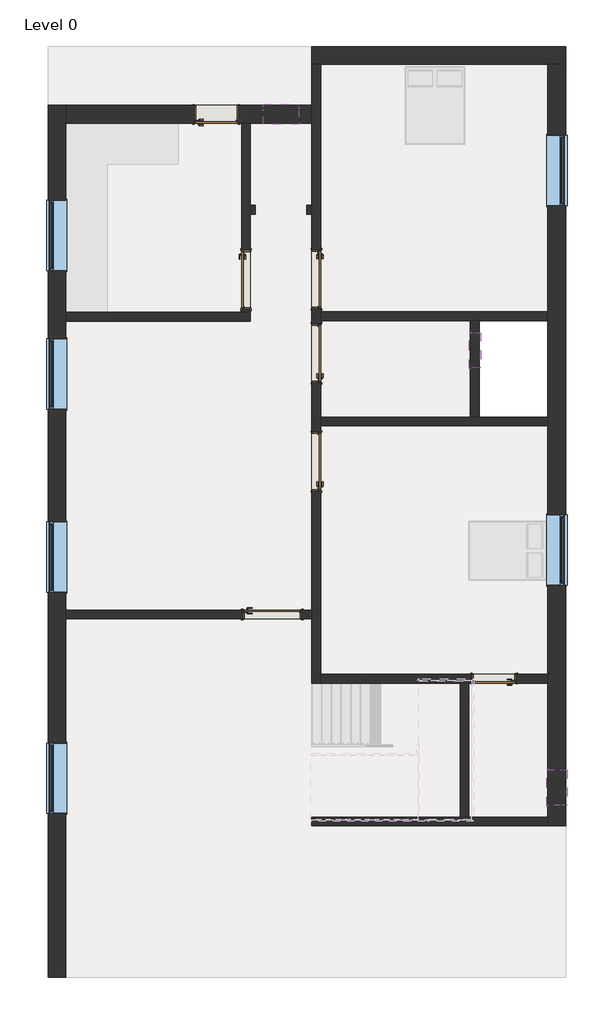
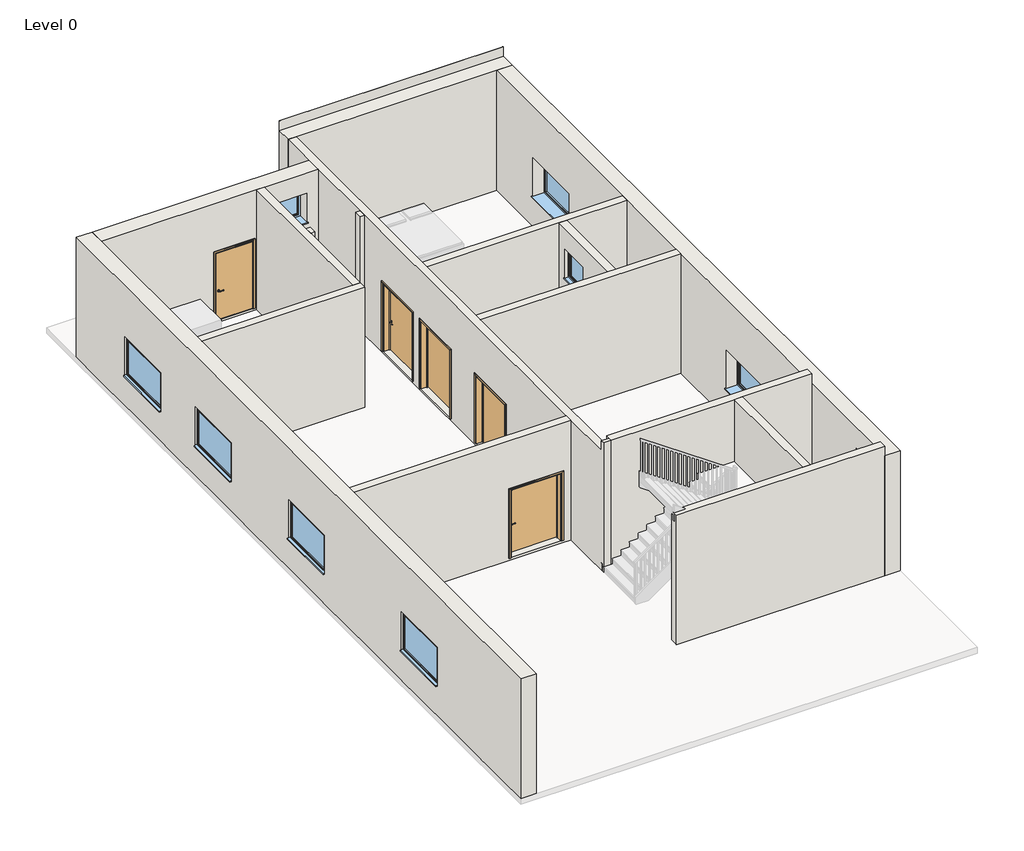
# One storey, part 1 of 2: 16 walls, 9 windows, 7 doors.
"""IFC4 building model written with IfcOpenShell, lengths in millimetres."""

from ifc_helpers import new_model, si_unit, frame, origin, origin_with_axes, place, context, project, spatial, polyline, outline, extrude, faceted_brep, transform, mapped, element, save
from components import doors_intsgl_d1_5c0f405e, doors_intsgl_d1_52b86bcf, doors_intsgl_d2_df50d10e, doors_intsgl_d2_875133e6, windows_sgl_plain_1810x1210mm_33e58113, windows_sgl_plain_1810x1210mm_8b4574cd, windows_sgl_plain_910x910mm_4715da24, windows_sgl_plain_910x910mm_27dc79fa, windows_sgl_plain_910x910mm_ba4b8fff

model = new_model("IFC4")

# Units and contexts
model_context = context("Model", 3, world=origin())
ifc_project = project(units=[si_unit("LENGTHUNIT", "METRE", prefix="MILLI")], contexts=[model_context])

# Site, building, storey
site = spatial("IfcSite", under=ifc_project)
building = spatial("IfcBuilding", under=site)
storey = spatial("IfcBuildingStorey", under=building, Name="Level 0", Elevation=0.0)

# Doors
placement = place(None, origin())
doors_intsgl_d1_shape = doors_intsgl_d1_5c0f405e(model_context)
element("IfcDoor", 1, ObjectType="Doors_IntSgl : D1", at=placement, inside=storey, context=model_context, shape_type="MappedRepresentation", body=[
    mapped(doors_intsgl_d1_shape, transform((-408.6988863, 5844.3566744, 76.2), x_axis=(0.0, -1.0, 0.0), y_axis=(1.0, 0.0, 0.0), z_axis=(0.0, 0.0, 1.0))),
])
element("IfcDoor", 2, ObjectType="Doors_IntSgl : D1", at=placement, inside=storey, context=model_context, shape_type="MappedRepresentation", body=[
    mapped(doors_intsgl_d1_shape, transform((-1538.9988863, -2784.8352742, 76.2), x_axis=(1.0, 0.0, 0.0), y_axis=(0.0, 1.0, 0.0), z_axis=(0.0, 0.0, 1.0))),
])
doors_intsgl_d1_2_shape = doors_intsgl_d1_52b86bcf(model_context)
element("IfcDoor", 3, ObjectType="Doors_IntSgl : D1", at=placement, inside=storey, context=model_context, shape_type="MappedRepresentation", body=[
    mapped(doors_intsgl_d1_2_shape, transform((-2218.4488863, 5838.4647258, 76.2), x_axis=(0.0, -1.0, 0.0), y_axis=(1.0, 0.0, 0.0), z_axis=(0.0, 0.0, 1.0))),
])
element("IfcDoor", 4, ObjectType="Doors_IntSgl : D1", at=placement, inside=storey, context=model_context, shape_type="MappedRepresentation", body=[
    mapped(doors_intsgl_d1_2_shape, transform((-408.6988863, 3939.3566744, 76.2), x_axis=(0.0, 1.0, 0.0), y_axis=(-1.0, 0.0, 0.0), z_axis=(0.0, 0.0, 1.0))),
])
element("IfcDoor", 5, ObjectType="Doors_IntSgl : D1", at=placement, inside=storey, context=model_context, shape_type="MappedRepresentation", body=[
    mapped(doors_intsgl_d1_2_shape, transform((-408.6988863, 1153.7809218, 76.2), x_axis=(0.0, 1.0, 0.0), y_axis=(-1.0, 0.0, 0.0), z_axis=(0.0, 0.0, 1.0))),
])
doors_intsgl_d2_shape = doors_intsgl_d2_df50d10e(model_context)
element("IfcDoor", 6, ObjectType="Doors_IntSgl : D2", at=placement, inside=storey, context=model_context, shape_type="MappedRepresentation", body=[
    mapped(doors_intsgl_d2_shape, transform((4169.6511137, -4435.8352742, 76.2), x_axis=(-1.0, 0.0, 0.0), y_axis=(0.0, -1.0, 0.0), z_axis=(0.0, 0.0, 1.0))),
])
doors_intsgl_d2_2_shape = doors_intsgl_d2_875133e6(model_context)
element("IfcDoor", 7, ObjectType="Doors_IntSgl : D2", at=placement, inside=storey, context=model_context, shape_type="MappedRepresentation", body=[
    mapped(doors_intsgl_d2_2_shape, transform((-2980.4488863, 10092.9647258, 76.2), x_axis=(1.0, 0.0, 0.0), y_axis=(0.0, 1.0, 0.0), z_axis=(0.0, 0.0, 1.0))),
])

# Walls
element("IfcWall", 8, ObjectType="EX WALL", at=placement, inside=storey, context=model_context, shape_type="Brep", body=[
    faceted_brep([(-7317.4988863, 10321.5647258, 0.0), (-7317.4988863, -12132.0352742, 0.0), (-7317.4988863, -12132.0352742, 3700.0), (-7317.4988863, 10321.5647258, 3700.0), (-7317.4988863, 7877.0647258, 2110.0), (-7317.4988863, 6067.0647258, 2110.0), (-7317.4988863, 6067.0647258, 900.0), (-7317.4988863, 7877.0647258, 900.0), (-7317.4988863, 4314.4647258, 2110.0), (-7317.4988863, 2504.4647258, 2110.0), (-7317.4988863, 2504.4647258, 900.0), (-7317.4988863, 4314.4647258, 900.0), (-7317.4988863, -403.3352742, 2110.0), (-7317.4988863, -2213.3352742, 2110.0), (-7317.4988863, -2213.3352742, 900.0), (-7317.4988863, -403.3352742, 900.0), (-7317.4988863, -6099.5352742, 2110.0), (-7317.4988863, -7909.5352742, 2110.0), (-7317.4988863, -7909.5352742, 900.0), (-7317.4988863, -6099.5352742, 900.0), (-6860.2988863, 10321.5647258, 0.0), (-6860.2988863, 10321.5647258, 3700.0), (-6860.2988863, 9864.3647258, 3700.0), (-6860.2988863, 5000.2647258, 3700.0), (-6860.2988863, 4771.6647258, 3700.0), (-6860.2988863, -2670.5352742, 3700.0), (-6860.2988863, -2899.1352742, 3700.0), (-6860.2988863, -12132.0352742, 3700.0), (-6860.2988863, -12132.0352742, 0.0), (-6860.2988863, -2899.1352742, 0.0), (-6860.2988863, -2670.5352742, 0.0), (-6860.2988863, 4771.6647258, 0.0), (-6860.2988863, 5000.2647258, 0.0), (-6860.2988863, 9864.3647258, 0.0), (-6860.2988863, 7877.0647258, 2110.0), (-6860.2988863, 7877.0647258, 900.0), (-6860.2988863, 6067.0647258, 900.0), (-6860.2988863, 6067.0647258, 2110.0), (-6860.2988863, 4314.4647258, 2110.0), (-6860.2988863, 4314.4647258, 900.0), (-6860.2988863, 2504.4647258, 900.0), (-6860.2988863, 2504.4647258, 2110.0), (-6860.2988863, -403.3352742, 2110.0), (-6860.2988863, -403.3352742, 900.0), (-6860.2988863, -2213.3352742, 900.0), (-6860.2988863, -2213.3352742, 2110.0), (-6860.2988863, -6099.5352742, 2110.0), (-6860.2988863, -6099.5352742, 900.0), (-6860.2988863, -7909.5352742, 900.0), (-6860.2988863, -7909.5352742, 2110.0)], [[[0, 1, 2, 3], [4, 5, 6, 7], [8, 9, 10, 11], [12, 13, 14, 15], [16, 17, 18, 19]], [[20, 21, 22, 23, 24, 25, 26, 27, 28, 29, 30, 31, 32, 33], [34, 35, 36, 37], [38, 39, 40, 41], [42, 43, 44, 45], [46, 47, 48, 49]], [[1, 0, 20, 33, 32, 31, 30, 29, 28]], [[2, 1, 28, 27]], [[0, 3, 21, 20]], [[3, 2, 27, 26, 25, 24, 23, 22, 21]], [[35, 34, 4, 7]], [[36, 35, 7, 6]], [[37, 36, 6, 5]], [[34, 37, 5, 4]], [[39, 38, 8, 11]], [[40, 39, 11, 10]], [[41, 40, 10, 9]], [[38, 41, 9, 8]], [[43, 42, 12, 15]], [[44, 43, 15, 14]], [[45, 44, 14, 13]], [[42, 45, 13, 12]], [[47, 46, 16, 19]], [[48, 47, 19, 18]], [[49, 48, 18, 17]], [[46, 49, 17, 16]]]),
])
element("IfcWall", 9, ObjectType="EX WALL", at=placement, inside=storey, context=model_context, shape_type="Brep", body=[
    faceted_brep([(-6860.2988863, 9864.3647258, 0.0), (-2332.7488863, 9864.3647258, 0.0), (-2104.1488863, 9864.3647258, 0.0), (-522.9988863, 9864.3647258, 0.0), (-522.9988863, 9864.3647258, 3700.0), (-2104.1488863, 9864.3647258, 3700.0), (-2332.7488863, 9864.3647258, 3700.0), (-6860.2988863, 9864.3647258, 3700.0), (-2408.9488863, 9864.3647258, 2186.2), (-2408.9488863, 9864.3647258, 76.2), (-3551.9488863, 9864.3647258, 76.2), (-3551.9488863, 9864.3647258, 2186.2), (-858.5738863, 9864.3647258, 3069.0), (-858.5738863, 9864.3647258, 2159.0), (-1768.5738863, 9864.3647258, 2159.0), (-1768.5738863, 9864.3647258, 3069.0), (-522.9988863, 10321.5647258, 0.0), (-6860.2988863, 10321.5647258, 0.0), (-6860.2988863, 10321.5647258, 3700.0), (-522.9988863, 10321.5647258, 3700.0), (-2408.9488863, 10321.5647258, 76.2), (-2408.9488863, 10321.5647258, 2186.2), (-3551.9488863, 10321.5647258, 2186.2), (-3551.9488863, 10321.5647258, 76.2), (-858.5738863, 10321.5647258, 3069.0), (-1768.5738863, 10321.5647258, 3069.0), (-1768.5738863, 10321.5647258, 2159.0), (-858.5738863, 10321.5647258, 2159.0)], [[[0, 1, 2, 3, 4, 5, 6, 7], [8, 9, 10, 11], [12, 13, 14, 15]], [[16, 17, 18, 19], [20, 21, 22, 23], [24, 25, 26, 27]], [[3, 2, 1, 0, 17, 16]], [[0, 7, 18, 17]], [[4, 3, 16, 19]], [[20, 9, 8, 21]], [[21, 8, 11, 22]], [[22, 11, 10, 23]], [[9, 20, 23, 10]], [[7, 6, 5, 4, 19, 18]], [[13, 12, 24, 27]], [[14, 13, 27, 26]], [[15, 14, 26, 25]], [[12, 15, 25, 24]]]),
])
element("IfcWall", 10, ObjectType="EX WALL", at=placement, inside=storey, context=model_context, shape_type="Brep", body=[
    faceted_brep([(-522.9988863, 11382.0147258, 0.0), (-294.3988863, 11382.0147258, 0.0), (5553.9511137, 11382.0147258, 0.0), (6011.1511137, 11382.0147258, 0.0), (6011.1511137, 11382.0147258, 3700.0), (5553.9511137, 11382.0147258, 3700.0), (-294.3988863, 11382.0147258, 3700.0), (-522.9988863, 11382.0147258, 3700.0), (-522.9988863, 11839.2147258, 0.0), (-522.9988863, 11839.2147258, 4000.0), (6011.1511137, 11839.2147258, 4000.0), (6011.1511137, 11839.2147258, 0.0), (6011.1511137, 11833.2891038, 4000.0), (6011.1511137, 11833.2891038, 3700.0), (-522.9988863, 11833.2891038, 3700.0), (-522.9988863, 11833.2891038, 4000.0)], [[[0, 1, 2, 3, 4, 5, 6, 7]], [[8, 9, 10, 11]], [[3, 2, 1, 0, 8, 11]], [[4, 3, 11, 10, 12, 13]], [[0, 7, 14, 15, 9, 8]], [[12, 10, 9, 15]], [[12, 15, 14, 13]], [[7, 6, 5, 4, 13, 14]]]),
])
element("IfcWall", 11, ObjectType="EX WALL", at=placement, inside=storey, context=model_context, shape_type="Brep", body=[
    faceted_brep([(5553.9511137, 11382.0147258, 0.0), (5553.9511137, 5006.1566744, 0.0), (5553.9511137, 4777.5566744, 0.0), (5553.9511137, 2296.7809218, 0.0), (5553.9511137, 2068.1809218, 0.0), (5553.9511137, -4321.5352742, 0.0), (5553.9511137, -4550.1352742, 0.0), (5553.9511137, -8002.321978, 0.0), (5553.9511137, -8230.921978, 0.0), (5553.9511137, -8230.921978, 3700.0), (5553.9511137, 2068.1809218, 3700.0), (5553.9511137, 2296.7809218, 3700.0), (5553.9511137, 4777.5566744, 3700.0), (5553.9511137, 5006.1566744, 3700.0), (5553.9511137, 11382.0147258, 3700.0), (5553.9511137, -2031.6771762, 2110.0), (5553.9511137, -2031.6771762, 900.0), (5553.9511137, -221.6771762, 900.0), (5553.9511137, -221.6771762, 2110.0), (5553.9511137, 9553.2147258, 2110.0), (5553.9511137, 7743.2147258, 2110.0), (5553.9511137, 7743.2147258, 900.0), (5553.9511137, 9553.2147258, 900.0), (5553.9511137, -6787.521978, 3069.0), (5553.9511137, -7697.521978, 3069.0), (5553.9511137, -7697.521978, 2159.0), (5553.9511137, -6787.521978, 2159.0), (6011.1511137, 11382.0147258, 0.0), (6011.1511137, 11382.0147258, 3700.0), (6011.1511137, -8230.921978, 3700.0), (6011.1511137, -8230.921978, 0.0), (6011.1511137, -2031.6771762, 2110.0), (6011.1511137, -221.6771762, 2110.0), (6011.1511137, -221.6771762, 900.0), (6011.1511137, -2031.6771762, 900.0), (6011.1511137, 9553.2147258, 2110.0), (6011.1511137, 9553.2147258, 900.0), (6011.1511137, 7743.2147258, 900.0), (6011.1511137, 7743.2147258, 2110.0), (6011.1511137, -6787.521978, 3069.0), (6011.1511137, -6787.521978, 2159.0), (6011.1511137, -7697.521978, 2159.0), (6011.1511137, -7697.521978, 3069.0)], [[[0, 1, 2, 3, 4, 5, 6, 7, 8, 9, 10, 11, 12, 13, 14], [15, 16, 17, 18], [19, 20, 21, 22], [23, 24, 25, 26]], [[27, 28, 29, 30], [31, 32, 33, 34], [35, 36, 37, 38], [39, 40, 41, 42]], [[8, 7, 6, 5, 4, 3, 2, 1, 0, 27, 30]], [[0, 14, 28, 27]], [[9, 8, 30, 29]], [[14, 13, 12, 11, 10, 9, 29, 28]], [[16, 15, 31, 34]], [[17, 16, 34, 33]], [[18, 17, 33, 32]], [[15, 18, 32, 31]], [[36, 35, 19, 22]], [[37, 36, 22, 21]], [[38, 37, 21, 20]], [[35, 38, 20, 19]], [[40, 39, 23, 26]], [[41, 40, 26, 25]], [[42, 41, 25, 24]], [[39, 42, 24, 23]]]),
])
element("IfcWall", 12, ObjectType="IN WALL", at=placement, inside=storey, context=model_context, shape_type="Brep", body=[
    faceted_brep([(-6860.2988863, 4771.6647258, 0.0), (-2104.1488863, 4771.6647258, 0.0), (-2104.1488863, 4771.6647258, 3700.0), (-6860.2988863, 4771.6647258, 3700.0), (-6860.2988863, 5000.2647258, 0.0), (-6860.2988863, 5000.2647258, 3700.0), (-2332.7488863, 5000.2647258, 3700.0), (-2104.1488863, 5000.2647258, 3700.0), (-2104.1488863, 5000.2647258, 0.0), (-2332.7488863, 5000.2647258, 0.0)], [[[0, 1, 2, 3]], [[4, 5, 6, 7, 8, 9]], [[1, 0, 4, 9, 8]], [[0, 3, 5, 4]], [[2, 1, 8, 7]], [[3, 2, 7, 6, 5]]]),
])
element("IfcWall", 13, ObjectType="IN WALL", at=placement, inside=storey, context=model_context, shape_type="Brep", body=[
    faceted_brep([(-2104.1488863, 5000.2647258, 0.0), (-2104.1488863, 7521.4694415, 0.0), (-2104.1488863, 7750.0694415, 0.0), (-2104.1488863, 9864.3647258, 0.0), (-2104.1488863, 9864.3647258, 3700.0), (-2104.1488863, 7750.0694415, 3700.0), (-2104.1488863, 7521.4694415, 3700.0), (-2104.1488863, 5000.2647258, 3700.0), (-2104.1488863, 5076.4647258, 76.2), (-2104.1488863, 5076.4647258, 2186.2), (-2104.1488863, 6600.4647258, 2186.2), (-2104.1488863, 6600.4647258, 76.2), (-2332.7488863, 9864.3647258, 0.0), (-2332.7488863, 5000.2647258, 0.0), (-2332.7488863, 5000.2647258, 3700.0), (-2332.7488863, 9864.3647258, 3700.0), (-2332.7488863, 5076.4647258, 2186.2), (-2332.7488863, 5076.4647258, 76.2), (-2332.7488863, 6600.4647258, 76.2), (-2332.7488863, 6600.4647258, 2186.2)], [[[0, 1, 2, 3, 4, 5, 6, 7], [8, 9, 10, 11]], [[12, 13, 14, 15], [16, 17, 18, 19]], [[3, 2, 1, 0, 13, 12]], [[0, 7, 14, 13]], [[4, 3, 12, 15]], [[8, 17, 16, 9]], [[9, 16, 19, 10]], [[10, 19, 18, 11]], [[17, 8, 11, 18]], [[7, 6, 5, 4, 15, 14]]]),
])
element("IfcWall", 14, ObjectType="IN WALL", at=placement, inside=storey, context=model_context, shape_type="Brep", body=[
    faceted_brep([(-522.9988863, 11382.0147258, 0.0), (-522.9988863, 10321.5647258, 0.0), (-522.9988863, 9864.3647258, 0.0), (-522.9988863, 7750.0694415, 0.0), (-522.9988863, 7521.4694415, 0.0), (-522.9988863, -2670.5352742, 0.0), (-522.9988863, -2899.1352742, 0.0), (-522.9988863, -4550.1352742, 0.0), (-522.9988863, -4550.1352742, 4000.0), (-522.9988863, -4436.6352742, 4000.0), (-522.9988863, -4436.6352742, 3700.0), (-522.9988863, -2899.1352742, 3700.0), (-522.9988863, -2670.5352742, 3700.0), (-522.9988863, 7521.4694415, 3700.0), (-522.9988863, 7750.0694415, 3700.0), (-522.9988863, 9864.3647258, 3700.0), (-522.9988863, 10321.5647258, 3700.0), (-522.9988863, 11382.0147258, 3700.0), (-522.9988863, 5082.3566744, 2186.2), (-522.9988863, 5082.3566744, 76.2), (-522.9988863, 6606.3566744, 76.2), (-522.9988863, 6606.3566744, 2186.2), (-522.9988863, 4701.3566744, 76.2), (-522.9988863, 4701.3566744, 2186.2), (-522.9988863, 3177.3566744, 2186.2), (-522.9988863, 3177.3566744, 76.2), (-522.9988863, 1915.7809218, 76.2), (-522.9988863, 1915.7809218, 2186.2), (-522.9988863, 391.7809218, 2186.2), (-522.9988863, 391.7809218, 76.2), (-294.3988863, -4550.1352742, 0.0), (-294.3988863, -4321.5352742, 0.0), (-294.3988863, 2068.1809218, 0.0), (-294.3988863, 2296.7809218, 0.0), (-294.3988863, 4777.5566744, 0.0), (-294.3988863, 5006.1566744, 0.0), (-294.3988863, 11382.0147258, 0.0), (-294.3988863, 11382.0147258, 3700.0), (-294.3988863, 5006.1566744, 3700.0), (-294.3988863, 4777.5566744, 3700.0), (-294.3988863, 2296.7809218, 3700.0), (-294.3988863, 2068.1809218, 3700.0), (-294.3988863, -4436.6352742, 3700.0), (-294.3988863, -4436.6352742, 4000.0), (-294.3988863, -4550.1352742, 4000.0), (-294.3988863, 5082.3566744, 76.2), (-294.3988863, 5082.3566744, 2186.2), (-294.3988863, 6606.3566744, 2186.2), (-294.3988863, 6606.3566744, 76.2), (-294.3988863, 4701.3566744, 2186.2), (-294.3988863, 4701.3566744, 76.2), (-294.3988863, 3177.3566744, 76.2), (-294.3988863, 3177.3566744, 2186.2), (-294.3988863, 1915.7809218, 2186.2), (-294.3988863, 1915.7809218, 76.2), (-294.3988863, 391.7809218, 76.2), (-294.3988863, 391.7809218, 2186.2)], [[[0, 1, 2, 3, 4, 5, 6, 7, 8, 9, 10, 11, 12, 13, 14, 15, 16, 17], [18, 19, 20, 21], [22, 23, 24, 25], [26, 27, 28, 29]], [[30, 31, 32, 33, 34, 35, 36, 37, 38, 39, 40, 41, 42, 43, 44], [45, 46, 47, 48], [49, 50, 51, 52], [53, 54, 55, 56]], [[7, 6, 5, 4, 3, 2, 1, 0, 36, 35, 34, 33, 32, 31, 30]], [[0, 17, 37, 36]], [[8, 7, 30, 44]], [[45, 19, 18, 46]], [[46, 18, 21, 47]], [[47, 21, 20, 48]], [[19, 45, 48, 20]], [[23, 22, 50, 49]], [[24, 23, 49, 52]], [[25, 24, 52, 51]], [[22, 25, 51, 50]], [[27, 26, 54, 53]], [[28, 27, 53, 56]], [[29, 28, 56, 55]], [[26, 29, 55, 54]], [[8, 44, 43, 9]], [[9, 43, 42, 10]], [[37, 17, 16, 15, 14, 13, 12, 11, 10, 42, 41, 40, 39, 38]]]),
])
element("IfcWall", 15, ObjectType="IN WALL", at=placement, inside=storey, context=model_context, shape_type="Brep", body=[
    faceted_brep([(-294.3988863, -4550.1352742, 0.0), (3293.3511137, -4550.1352742, 0.0), (3521.9511137, -4550.1352742, 0.0), (5553.9511137, -4550.1352742, 0.0), (5553.9511137, -4550.1352742, 4000.0), (3521.6011137, -4550.1352742, 4000.0), (3293.3511137, -4550.1352742, 4000.0), (-294.3988863, -4550.1352742, 4000.0), (3598.1511137, -4550.1352742, 76.2), (3598.1511137, -4550.1352742, 2186.2), (4741.1511137, -4550.1352742, 2186.2), (4741.1511137, -4550.1352742, 76.2), (5553.9511137, -4321.5352742, 0.0), (-294.3988863, -4321.5352742, 0.0), (-294.3988863, -4321.5352742, 4000.0), (5553.9511137, -4321.5352742, 4000.0), (3598.1511137, -4321.5352742, 2186.2), (3598.1511137, -4321.5352742, 76.2), (4741.1511137, -4321.5352742, 76.2), (4741.1511137, -4321.5352742, 2186.2), (-294.3988863, -4436.6352742, 4000.0)], [[[0, 1, 2, 3, 4, 5, 6, 7], [8, 9, 10, 11]], [[12, 13, 14, 15], [16, 17, 18, 19]], [[3, 2, 1, 0, 13, 12]], [[7, 6, 5, 4, 15, 14, 20]], [[0, 7, 20, 14, 13]], [[4, 3, 12, 15]], [[8, 17, 16, 9]], [[9, 16, 19, 10]], [[10, 19, 18, 11]], [[17, 8, 11, 18]]]),
])
element("IfcWall", 16, ObjectType="IN WALL", at=placement, inside=storey, context=model_context, shape_type="Brep", body=[
    faceted_brep([(-520.2140986, -8230.921978, 0.0), (5553.9511137, -8230.921978, 0.0), (5553.9511137, -8230.921978, 3700.0), (5553.9511137, -8230.921978, 4000.0), (-520.2140986, -8230.921978, 4000.0), (-520.2140986, -8002.321978, 0.0), (-520.2140986, -8002.321978, 4000.0), (3293.3511137, -8002.321978, 4000.0), (3521.6011137, -8002.321978, 4000.0), (5553.9511137, -8002.321978, 4000.0), (5553.9511137, -8002.321978, 0.0), (3521.9511137, -8002.321978, 0.0), (3293.3511137, -8002.321978, 0.0)], [[[0, 1, 2, 3, 4]], [[5, 6, 7, 8, 9, 10, 11, 12]], [[1, 0, 5, 12, 11, 10]], [[4, 3, 9, 8, 7, 6]], [[0, 4, 6, 5]], [[3, 2, 1, 10, 9]]]),
])
element("IfcWall", 17, ObjectType="IN WALL", at=placement, inside=storey, context=model_context, shape_type="SweptSolid", body=[
    extrude(outline(polyline([(4000.0, 3293.3511137), (0.0, 3293.3511137), (0.0, 3521.9511137), (3700.0, 3521.9511137), (3700.0, 3521.6011137), (4000.0, 3521.6011137), (4000.0, 3293.3511137)])), frame((0.0, -8002.321978, 0.0), z_axis=(0.0, 1.0, 0.0), x_axis=(0.0, 0.0, 1.0)), (0.0, 0.0, 1.0), 3452.1867039),
])
element("IfcWall", 18, ObjectType="IN WALL", at=placement, inside=storey, context=model_context, shape_type="SweptSolid", body=[
    extrude(outline(polyline([(0.0, -6860.2988863), (0.0, -522.9988863), (3700.0, -522.9988863), (3700.0, -6860.2988863), (0.0, -6860.2988863)]), holes=[polyline([(2186.2, -776.9988863), (76.2, -776.9988863), (76.2, -2300.9988863), (2186.2, -2300.9988863), (2186.2, -776.9988863)])]), frame((0.0, -2899.1352742, 0.0), z_axis=(0.0, 1.0, 0.0), x_axis=(0.0, 0.0, 1.0)), (0.0, 0.0, 1.0), 228.6),
])
element("IfcWall", 19, ObjectType="IN WALL", at=placement, inside=storey, context=model_context, shape_type="Brep", body=[
    faceted_brep([(-294.3988863, 4777.5566744, 0.0), (3560.0511137, 4777.5566744, 0.0), (3788.6511137, 4777.5566744, 0.0), (5553.9511137, 4777.5566744, 0.0), (5553.9511137, 4777.5566744, 3700.0), (3788.6511137, 4777.5566744, 3700.0), (3560.0511137, 4777.5566744, 3700.0), (-294.3988863, 4777.5566744, 3700.0), (-294.3988863, 5006.1566744, 0.0), (-294.3988863, 5006.1566744, 3700.0), (5553.9511137, 5006.1566744, 3700.0), (5553.9511137, 5006.1566744, 0.0)], [[[0, 1, 2, 3, 4, 5, 6, 7]], [[8, 9, 10, 11]], [[3, 2, 1, 0, 8, 11]], [[4, 3, 11, 10]], [[0, 7, 9, 8]], [[7, 6, 5, 4, 10, 9]]]),
])
element("IfcWall", 20, ObjectType="IN WALL", at=placement, inside=storey, context=model_context, shape_type="Brep", body=[
    faceted_brep([(-294.3988863, 2068.1809218, 0.0), (5553.9511137, 2068.1809218, 0.0), (5553.9511137, 2068.1809218, 3700.0), (-294.3988863, 2068.1809218, 3700.0), (-294.3988863, 2296.7809218, 0.0), (-294.3988863, 2296.7809218, 3700.0), (3560.0511137, 2296.7809218, 3700.0), (3788.6511137, 2296.7809218, 3700.0), (5553.9511137, 2296.7809218, 3700.0), (5553.9511137, 2296.7809218, 0.0), (3788.6511137, 2296.7809218, 0.0), (3560.0511137, 2296.7809218, 0.0)], [[[0, 1, 2, 3]], [[4, 5, 6, 7, 8, 9, 10, 11]], [[1, 0, 4, 11, 10, 9]], [[2, 1, 9, 8]], [[0, 3, 5, 4]], [[3, 2, 8, 7, 6, 5]]]),
])
element("IfcWall", 21, ObjectType="IN WALL", at=placement, inside=storey, context=model_context, shape_type="SweptSolid", body=[
    extrude(outline(polyline([(4777.5566744, 0.0), (2296.7809218, 0.0), (2296.7809218, 3700.0), (4777.5566744, 3700.0), (4777.5566744, 0.0)]), holes=[polyline([(4472.7566744, 3069.0), (3562.7566744, 3069.0), (3562.7566744, 2159.0), (4472.7566744, 2159.0), (4472.7566744, 3069.0)])]), frame((3560.0511137, 0.0, 0.0), z_axis=(1.0, 0.0, 0.0), x_axis=(0.0, 1.0, 0.0)), (0.0, 0.0, 1.0), 228.6),
])
element("IfcWall", 22, ObjectType="IN WALL", at=placement, inside=storey, context=model_context, shape_type="SweptSolid", body=[
    extrude(outline(polyline([(-1977.1488863, 7521.4694415), (-2104.1488863, 7521.4694415), (-2104.1488863, 7750.0694415), (-1977.1488863, 7750.0694415), (-1977.1488863, 7521.4694415)])), origin_with_axes(), (0.0, 0.0, 1.0), 3700.0),
])
element("IfcWall", 23, ObjectType="IN WALL", at=placement, inside=storey, context=model_context, shape_type="SweptSolid", body=[
    extrude(outline(polyline([(-522.9988863, 7521.4694415), (-649.9988863, 7521.4694415), (-649.9988863, 7750.0694415), (-522.9988863, 7750.0694415), (-522.9988863, 7521.4694415)])), origin_with_axes(), (0.0, 0.0, 1.0), 3700.0),
])

# Windows
windows_sgl_plain_1810x1210mm_shape = windows_sgl_plain_1810x1210mm_33e58113(model_context)
element("IfcWindow", 24, ObjectType="Windows_Sgl_Plain : 1810x1210mm", at=placement, inside=storey, context=model_context, shape_type="MappedRepresentation", body=[
    mapped(windows_sgl_plain_1810x1210mm_shape, transform((5774.0945459, 8648.2147258, 0.0), x_axis=(0.0, -1.0, 0.0), y_axis=(1.0, 0.0, 0.0), z_axis=(0.0, 0.0, 1.0))),
])
windows_sgl_plain_1810x1210mm_2_shape = windows_sgl_plain_1810x1210mm_8b4574cd(model_context)
element("IfcWindow", 25, ObjectType="Windows_Sgl_Plain : 1810x1210mm", at=placement, inside=storey, context=model_context, shape_type="MappedRepresentation", body=[
    mapped(windows_sgl_plain_1810x1210mm_2_shape, transform((-7080.4423185, 6972.0647258, 0.0), x_axis=(0.0, -1.0, 0.0), y_axis=(1.0, 0.0, 0.0), z_axis=(0.0, 0.0, 1.0))),
])
element("IfcWindow", 26, ObjectType="Windows_Sgl_Plain : 1810x1210mm", at=placement, inside=storey, context=model_context, shape_type="MappedRepresentation", body=[
    mapped(windows_sgl_plain_1810x1210mm_2_shape, transform((-7080.4423185, 3409.4647258, 0.0), x_axis=(0.0, -1.0, 0.0), y_axis=(1.0, 0.0, 0.0), z_axis=(0.0, 0.0, 1.0))),
])
element("IfcWindow", 27, ObjectType="Windows_Sgl_Plain : 1810x1210mm", at=placement, inside=storey, context=model_context, shape_type="MappedRepresentation", body=[
    mapped(windows_sgl_plain_1810x1210mm_2_shape, transform((-7080.4423185, -1308.3352742, 0.0), x_axis=(0.0, -1.0, 0.0), y_axis=(1.0, 0.0, 0.0), z_axis=(0.0, 0.0, 1.0))),
])
element("IfcWindow", 28, ObjectType="Windows_Sgl_Plain : 1810x1210mm", at=placement, inside=storey, context=model_context, shape_type="MappedRepresentation", body=[
    mapped(windows_sgl_plain_1810x1210mm_2_shape, transform((-7080.4423185, -7004.5352742, 0.0), x_axis=(0.0, -1.0, 0.0), y_axis=(1.0, 0.0, 0.0), z_axis=(0.0, 0.0, 1.0))),
])
element("IfcWindow", 29, ObjectType="Windows_Sgl_Plain : 1810x1210mm", at=placement, inside=storey, context=model_context, shape_type="MappedRepresentation", body=[
    mapped(windows_sgl_plain_1810x1210mm_2_shape, transform((5774.0945459, -1126.6771762, 0.0), x_axis=(0.0, 1.0, 0.0), y_axis=(-1.0, 0.0, 0.0), z_axis=(0.0, 0.0, 1.0))),
])
windows_sgl_plain_910x910mm_shape = windows_sgl_plain_910x910mm_4715da24(model_context)
element("IfcWindow", 30, ObjectType="Windows_Sgl_Plain : 910x910mm", at=placement, inside=storey, context=model_context, shape_type="MappedRepresentation", body=[
    mapped(windows_sgl_plain_910x910mm_shape, transform((5774.0945459, -7242.521978, 959.0), x_axis=(0.0, -1.0, 0.0), y_axis=(1.0, 0.0, 0.0), z_axis=(0.0, 0.0, 1.0))),
])
windows_sgl_plain_910x910mm_2_shape = windows_sgl_plain_910x910mm_27dc79fa(model_context)
element("IfcWindow", 31, ObjectType="Windows_Sgl_Plain : 910x910mm", at=placement, inside=storey, context=model_context, shape_type="MappedRepresentation", body=[
    mapped(windows_sgl_plain_910x910mm_2_shape, transform((-1313.5738863, 10084.508158, 959.0), x_axis=(-1.0, 0.0, 0.0), y_axis=(0.0, -1.0, 0.0), z_axis=(0.0, 0.0, 1.0))),
])
windows_sgl_plain_910x910mm_3_shape = windows_sgl_plain_910x910mm_ba4b8fff(model_context)
element("IfcWindow", 32, ObjectType="Windows_Sgl_Plain : 910x910mm", at=placement, inside=storey, context=model_context, shape_type="MappedRepresentation", body=[
    mapped(windows_sgl_plain_910x910mm_3_shape, transform((3665.8945459, 4017.7566744, 959.0), x_axis=(0.0, -1.0, 0.0), y_axis=(1.0, 0.0, 0.0), z_axis=(0.0, 0.0, 1.0))),
])

save(model, "model.ifc")

# Revit data of these elements
# Type "Doors_IntSgl : D1"
#   Type Mark = "46"
#   Type Comments = "Internal Single"
#   Operation = "SingleSwingRight"
#   Manufacturer = "Revit"
#   Keynote = "L20"
#   Description = "Internal Single Door"
#   Analytic Construction = "Metal"
#   UnderCut = 8 mm
#   Tolerance = 2 mm
#   Thickness = 38 mm
#   Thermal Resistance (R) = 0.270117 (m²·K)/W
#   Structural Tolerance = 8 mm
#   StopDepth = 32 mm
#   Stop Thickness = 19 mm
#   Rough Width = 1524 mm
#   Rough Height = 2110 mm
#   Height to Top Lock Rail = 1000 mm
#   Heat Transfer Coefficient (U) = 3.7021 W/(m²·K)
#   Handle Z Distance = 900 mm
#   Handle X Distance = 75 mm
#   Frame Thickness = 32 mm
#   Door Panel Width = 1440 mm
#   Door Panel Thickness = 38 mm
#   Door Panel Offset = 0 mm
#   Height = 2110 mm
#   Width = 1524 mm
#   Door Panel Height = 2060 mm
#   Architrave Setback = 5 mm
#   Vis - Ironmongery = yes
#   Material Ironmongery = Door - Handle
#   Material Frame = Door - Frame/Mullion (1)
#   Material Door = Door - Panel
#   Material Architrave = Door - Architrave
#   Visual Light Transmittance = 0
#   Solar Heat Gain Coefficient = 0
#   Function = (empty or 0)
#   Wall Closure = (empty or 0)
# Type "Doors_IntSgl : D2"
#   Type Mark = "47"
#   Type Comments = "Internal Single"
#   Operation = "SingleSwingRight"
#   Manufacturer = "Revit"
#   Keynote = "L20"
#   Description = "Internal Single Door"
#   Analytic Construction = "Metal"
#   UnderCut = 8 mm
#   Tolerance = 2 mm
#   Thickness = 38 mm
#   Thermal Resistance (R) = 0.270117 (m²·K)/W
#   Structural Tolerance = 8 mm
#   StopDepth = 32 mm
#   Stop Thickness = 19 mm
#   Rough Width = 1143 mm
#   Rough Height = 2110 mm
#   Height to Top Lock Rail = 1000 mm
#   Heat Transfer Coefficient (U) = 3.7021 W/(m²·K)
#   Handle Z Distance = 900 mm
#   Handle X Distance = 75 mm
#   Frame Thickness = 32 mm
#   Door Panel Width = 1059 mm
#   Door Panel Thickness = 38 mm
#   Door Panel Offset = 0 mm
#   Height = 2110 mm
#   Width = 1143 mm
#   Door Panel Height = 2060 mm
#   Architrave Setback = 5 mm
#   Vis - Ironmongery = yes
#   Material Ironmongery = Door - Handle
#   Material Frame = Door - Frame/Mullion (1)
#   Material Door = Door - Panel
#   Material Architrave = Door - Architrave
#   Visual Light Transmittance = 0
#   Solar Heat Gain Coefficient = 0
#   Function = (empty or 0)
#   Wall Closure = (empty or 0)
# Type "EX WALL"
#   Keynote = "F10"
#   Layers, outside or top first: 457.2 mm "Concrete Masonry Units _Low Density" (function 1)
# Type "IN WALL"
#   Keynote = "F10"
#   Layers, outside or top first: 228.6 mm "Concrete Masonry Units _Low Density" (function 1)
# Type "Windows_Sgl_Plain : 1810x1210mm"
#   Type Mark = "49"
#   Operation = "SinglePanel"
#   Construction Type Id = "SGL"
#   Manufacturer = "Revit"
#   Keynote = "L10"
#   Analytic Construction = "Large single-glazed windows"
#   Wrap Layers (Ext) from Ext = 102.5 mm
#   Wrap Layers (Int) from Ext = 177.5 mm
#   Window Board Projection = 25 mm
#   Window Board Extension = 25 mm
#   Visual Light Transmittance = 0.9
#   Solar Heat Gain Coefficient = 0.86
#   Rough Width = 1810 mm
#   Rough Height = 1210 mm
#   Height = 1210 mm
#   Width = 1810 mm
#   Heat Transfer Coefficient (U) = 5.5617 W/(m²·K)
#   Glazing Thickness = 24 mm
#   FrameOffset - External = 50 mm
#   Frame Depth = 65 mm
#   Default Head Height = 2110 mm
#   Cill Depth = 87.5 mm
#   Cavity Closer Width = 50 mm
#   Cavity Closer Offset from Ext = 102.5 mm
#   Cavity Closer Depth = 85 mm
#   Define Thermal Properties by = 1
#   Vis - Cavity Closers = yes
#   Define Thermal Properties by = 1
#   Material Trim = Window Frame
#   Material Glass = Glass
#   Material Frame = Window Frame
#   Wall Closure = (empty or 0)
# Type "Windows_Sgl_Plain : 910x910mm"
#   Type Mark = "44"
#   Operation = "SinglePanel"
#   Construction Type Id = "SGL"
#   Manufacturer = "Revit"
#   Keynote = "L10"
#   Analytic Construction = "Large single-glazed windows"
#   Wrap Layers (Ext) from Ext = 102.5 mm
#   Wrap Layers (Int) from Ext = 177.5 mm
#   Window Board Projection = 25 mm
#   Window Board Extension = 25 mm
#   Visual Light Transmittance = 0.9
#   Solar Heat Gain Coefficient = 0.86
#   Rough Width = 910 mm
#   Rough Height = 910 mm
#   Height = 910 mm
#   Width = 910 mm
#   Heat Transfer Coefficient (U) = 5.5617 W/(m²·K)
#   Glazing Thickness = 24 mm
#   FrameOffset - External = 50 mm
#   Frame Depth = 65 mm
#   Default Head Height = 2110 mm
#   Cill Depth = 87.5 mm
#   Cavity Closer Width = 50 mm
#   Cavity Closer Offset from Ext = 102.5 mm
#   Cavity Closer Depth = 85 mm
#   Define Thermal Properties by = 1
#   Vis - Cavity Closers = yes
#   Define Thermal Properties by = 1
#   Material Trim = Window Frame
#   Material Glass = Glass
#   Material Frame = Window Frame
#   Wall Closure = (empty or 0)
# Elements 1, 2, 3, 4, 5 (IfcDoor, "Doors_IntSgl : D1")
#   Phase Created = New Construction
#   Materials on its faces: "Door - Architrave", "Door - Handle", "Door - Frame/Mullion (1)", "Door - Panel"
# Elements 6, 7 (IfcDoor, "Doors_IntSgl : D2")
#   Phase Created = New Construction
#   Materials on its faces: "Door - Architrave", "Door - Handle", "Door - Frame/Mullion (1)", "Door - Panel"
# Elements 8, 9, 10, 11 (IfcWall, "EX WALL")
#   Top Offset = 0 mm
#   Base Offset = 0 mm
#   wall height = 4000 mm
#   Phase Created = New Construction
#   Base Constraint = Level 0
#   Top Constraint = Level 1
#   Materials on its faces: "Concrete Masonry Units _Low Density"
# Elements 12, 13, 14, 15, 16, 17, 18, 19, 20, 21, 22, 23 (IfcWall, "IN WALL")
#   Top Offset = 0 mm
#   Base Offset = 0 mm
#   wall height = 4000 mm
#   Phase Created = New Construction
#   Base Constraint = Level 0
#   Top Constraint = Level 1
#   Materials on its faces: "Concrete Masonry Units _Low Density"
# Element 24 (IfcWindow, "Windows_Sgl_Plain : 1810x1210mm")
#   Mark = "6"
#   Phase Created = New Construction
#   Materials on its faces: "Window Frame", "Glass"
# Element 25 (IfcWindow, "Windows_Sgl_Plain : 1810x1210mm")
#   Mark = "1"
#   Phase Created = New Construction
#   Materials on its faces: "Window Frame", "Glass"
# Element 26 (IfcWindow, "Windows_Sgl_Plain : 1810x1210mm")
#   Mark = "2"
#   Phase Created = New Construction
#   Materials on its faces: "Window Frame", "Glass"
# Element 27 (IfcWindow, "Windows_Sgl_Plain : 1810x1210mm")
#   Mark = "3"
#   Phase Created = New Construction
#   Materials on its faces: "Window Frame", "Glass"
# Element 28 (IfcWindow, "Windows_Sgl_Plain : 1810x1210mm")
#   Mark = "4"
#   Phase Created = New Construction
#   Materials on its faces: "Window Frame", "Glass"
# Element 29 (IfcWindow, "Windows_Sgl_Plain : 1810x1210mm")
#   Mark = "5"
#   Phase Created = New Construction
#   Materials on its faces: "Window Frame", "Glass"
# Element 30 (IfcWindow, "Windows_Sgl_Plain : 910x910mm")
#   Mark = "8"
#   Phase Created = New Construction
#   Materials on its faces: "Window Frame", "Glass"
# Element 31 (IfcWindow, "Windows_Sgl_Plain : 910x910mm")
#   Mark = "7"
#   Phase Created = New Construction
#   Materials on its faces: "Window Frame", "Glass"
# Element 32 (IfcWindow, "Windows_Sgl_Plain : 910x910mm")
#   Mark = "9"
#   Phase Created = New Construction
#   Materials on its faces: "Window Frame", "Glass"
# Materials
#   "Door - Handle": colour RGB 0 0 0, transparency 0, Keynote = "P21", Cost = 0
#   "Door - Frame/Mullion (1)": class "Wood", colour RGB 212 179 113, transparency 0, Keynote = "L20", Cost = 0
#   "Door - Panel": class "Wood", colour RGB 210 159 95, transparency 0, Keynote = "L20", Cost = 0
#   "Door - Architrave": class "Wood", colour RGB 154 90 5, transparency 0, Keynote = "P20", Cost = 0
#   "Concrete Masonry Units _Low Density": class "Masonry", colour RGB 181 181 181, transparency 0, Description = "Concrete masonry units", Cost = 0
#   "Window Frame": colour RGB 249 249 249, transparency 0, Keynote = "L10", Cost = 0
#   "Glass": class "Glass", colour RGB 0 128 192, transparency 0.9, Description = "Soda Lime Glass", Cost = 0
# Room at (4545.224, -6189.837) mm, phase "New Construction", upper level "Level 0", upper offset 3999.992 mm, lower offset 0 mm
#   Number = "8"
#   Name = "toilet 2"
# Room at (-4313.75, 7572.957) mm, phase "New Construction", upper level "Level 0", upper offset 3999.992 mm, lower offset 0 mm
#   Number = "1"
#   Name = "kitchen"
# Room at (-3301.75, 945.757) mm, phase "New Construction", upper level "Level 0", upper offset 3999.992 mm, lower offset 0 mm
#   Number = "2"
#   Name = "hall"
# Room at (-1317.478, 8797.588) mm, phase "New Construction", upper level "Level 0", upper offset 3999.992 mm, lower offset 0 mm
#   Number = "3"
# Room at (2086.767, 8020.666) mm, phase "New Construction", upper level "Level 0", upper offset 3999.992 mm, lower offset 0 mm
#   Number = "4"
#   Name = "bed room 1"
# Room at (2086.767, 3313.927) mm, phase "New Construction", upper level "Level 0", upper offset 3999.992 mm, lower offset 0 mm
#   Number = "5"
#   Name = "toilet 1"
# Room at (3098.767, -1215.199) mm, phase "New Construction", upper level "Level 0", upper offset 3999.992 mm, lower offset 0 mm
#   Number = "6"
#   Name = "bed room 2"
# Room, not placed, phase "New Construction", upper offset 0 mm, lower offset 0 mm
#   Number = "7"
#   Name = "open area"
# Room at (3069.267, -10259.783) mm, phase "New Construction", upper level "Level 0", upper offset 3999.992 mm, lower offset 0 mm
#   Number = "10"
#   Name = "Room"
# Room at (-3506.25, -8278.853) mm, phase "New Construction", upper level "Level 0", upper offset 3999.992 mm, lower offset 0 mm
#   Number = "9"
#   Name = "parking"
